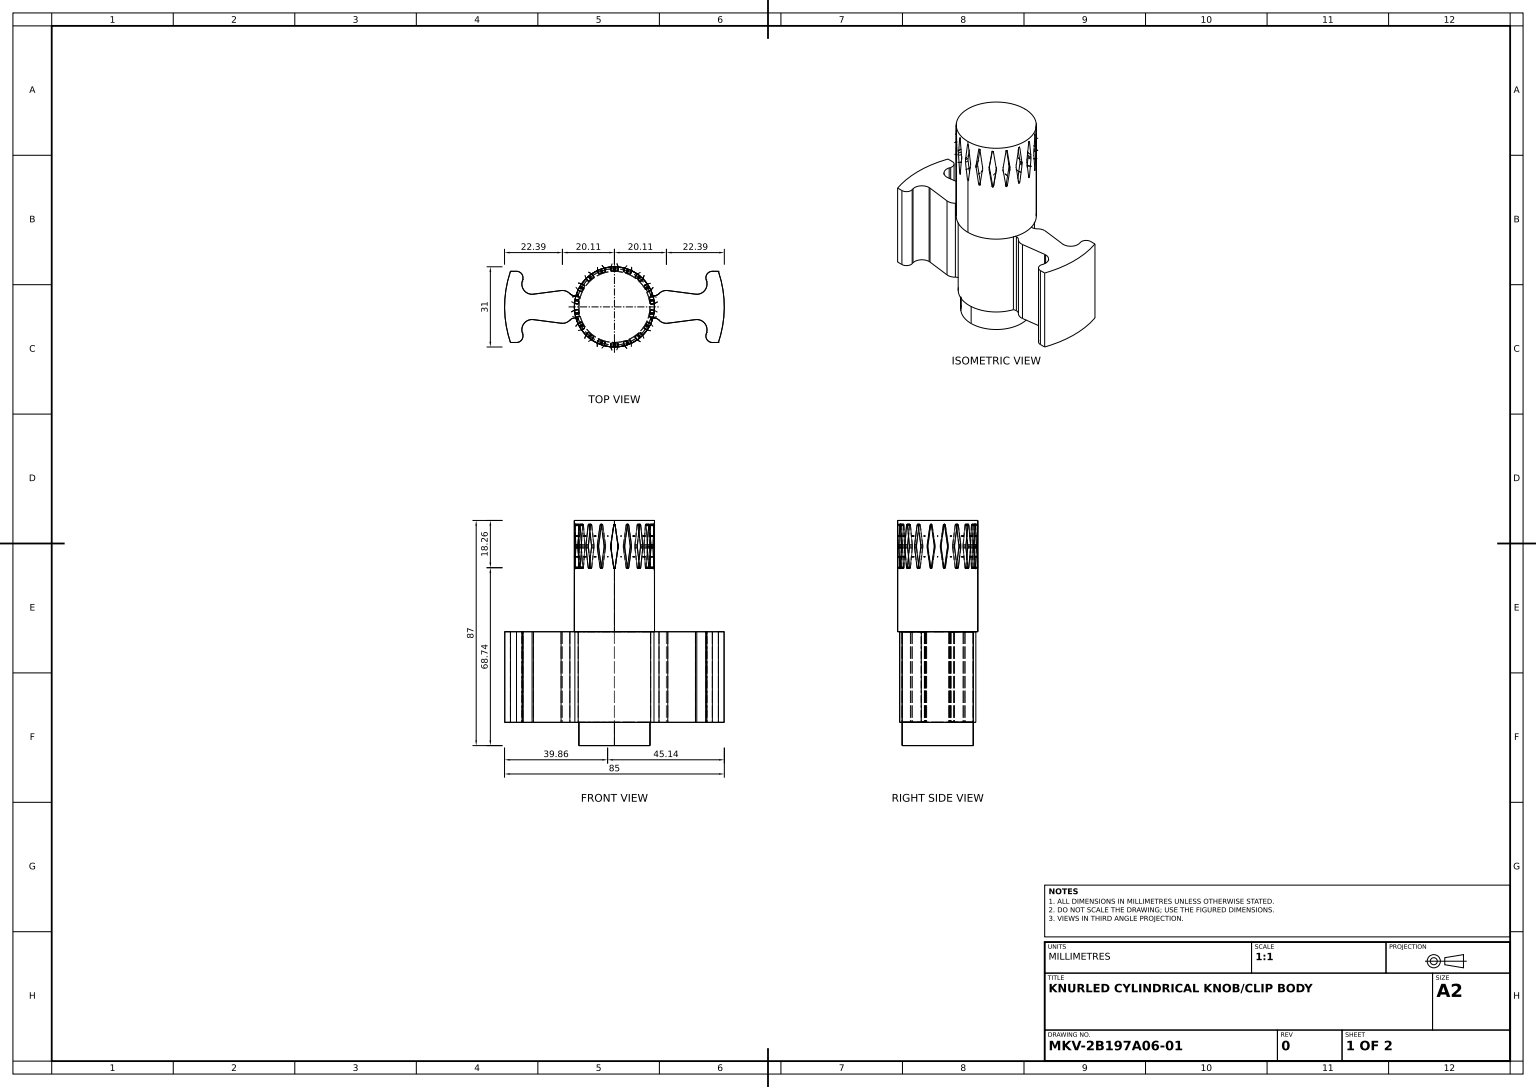
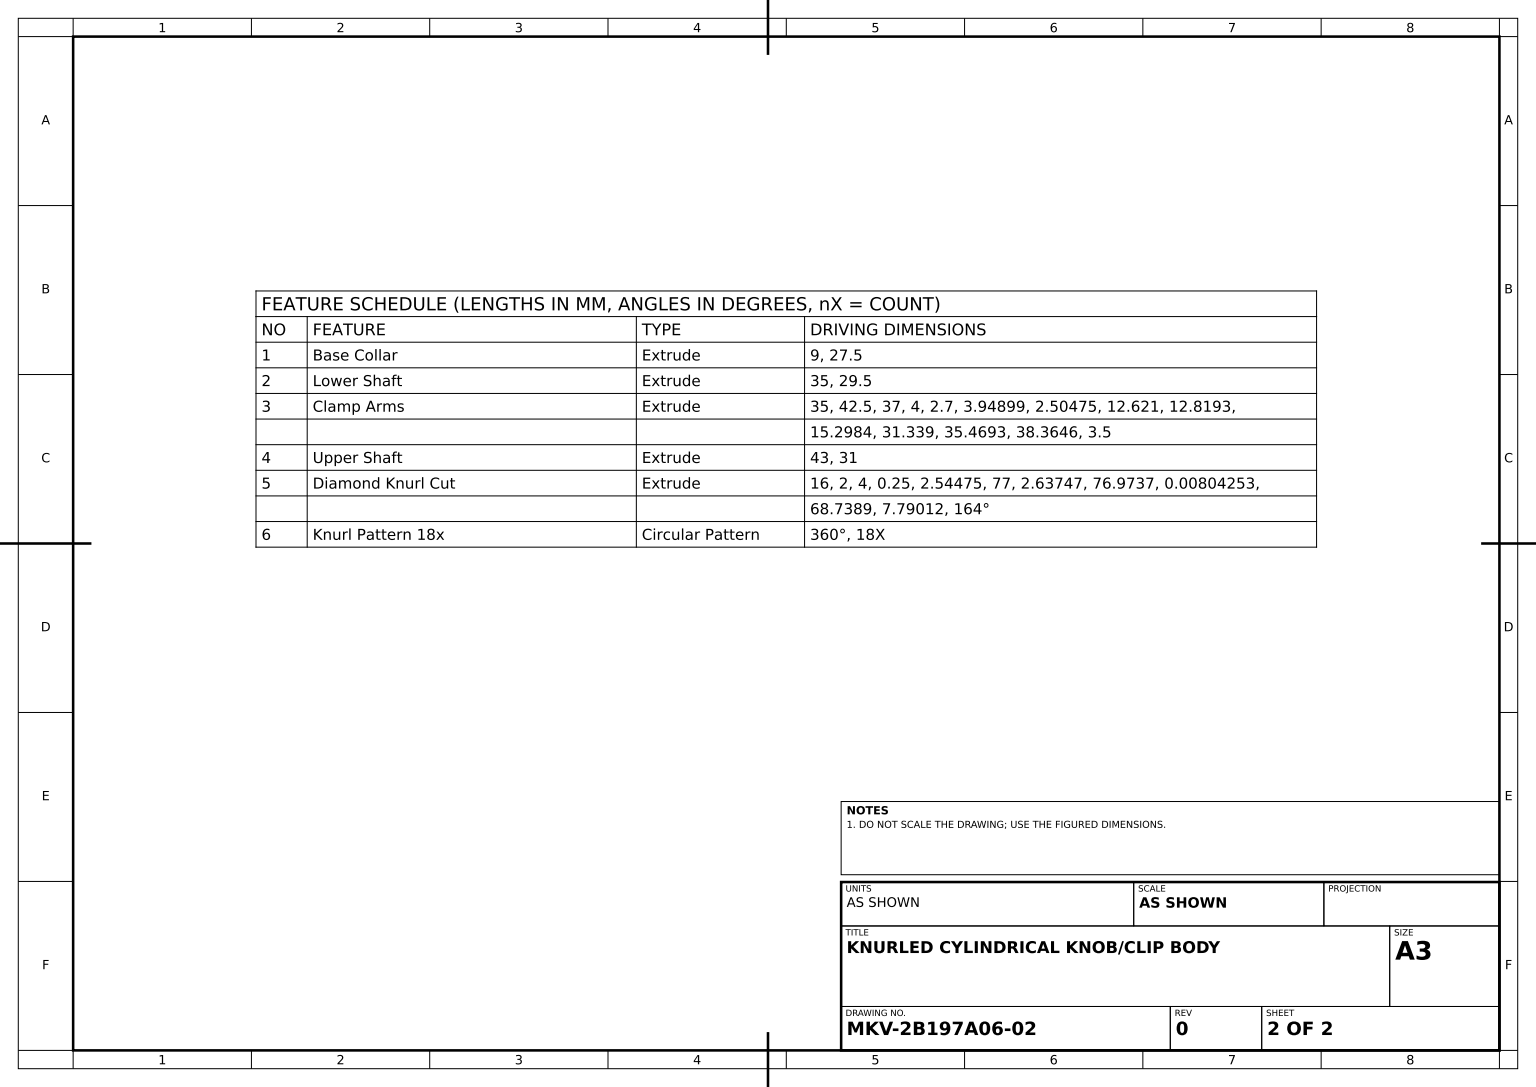
from build123d import *

# Parameters (mm, degrees)
BASE_COLLAR_SKETCH_R    = 13.75
BASE_COLLAR_DEPTH       = 9
LOWER_SHAFT_SKETCH_R    = 14.75
LOWER_SHAFT_DEPTH       = 35
CLAMP_ARMS_DEPTH        = 35
UPPER_SHAFT_SKETCH_R    = 15.5
UPPER_SHAFT_DEPTH       = 43
DIAMOND_KNURL_CUT_DEPTH = 2
KNURL_PATTERN_18X_COUNT = 18


with BuildPart() as part:
    # Base Collar Sketch → Base Collar (new body)
    with BuildSketch(Plane(origin=(0, 0, 0), x_dir=(1, 0, 0), z_dir=(0, 1, 0))):
        with Locations(Location((0, 0, 0), (0, 0, 270))):
            Circle(BASE_COLLAR_SKETCH_R)
    extrude(amount=BASE_COLLAR_DEPTH)

    # Lower Shaft Sketch → Lower Shaft (add)
    with BuildSketch(Plane(origin=(0, 9, 0), x_dir=(1, 0, 0), z_dir=(0, 1, 0))):
        with Locations(Location((0, 0, 0), (0, 0, 270))):
            Circle(LOWER_SHAFT_SKETCH_R)
    extrude(amount=LOWER_SHAFT_DEPTH)

    # Clamp Arms Sketch → Clamp Arms (add)
    with BuildSketch(Plane.XZ.offset(-9)):
        with BuildLine():
            Line((37.870431389, -13.75), (40.214269855, -13.75))
            ThreePointArc((40.214269855, -13.75), (42.5, 0), (40.214269855, 13.75))
            Line((40.214269855, 13.75), (37.870431389, 13.75))
            ThreePointArc((37.870431389, 13.75), (35.862990958, 12.743233464), (35.469303802, 10.532259389))
            ThreePointArc((35.469303802, 10.532259389), (35.563515946, 10.209619659), (35.654793325, 9.886137414))
            ThreePointArc((35.654793325, 9.886137414), (34.831320299, 6.242068845), (31.338961442, 4.915127559))
            Line((31.338961442, 4.915127559), (20.628220903, 6.311217501))
            ThreePointArc((20.628220903, 6.311217501), (18.792751829, 6.121230791), (17.237871609, 5.127556211))
            ThreePointArc((17.237871609, 5.127556211), (15.702646269, 4.336375699), (14.001999226, 4.637512015))
            ThreePointArc((14.001999226, 4.637512015), (14.75, 0), (14.001999226, -4.637512015))
            ThreePointArc((14.001999226, -4.637512015), (15.702646269, -4.336375699), (17.237871609, -5.127556211))
            ThreePointArc((17.237871609, -5.127556211), (18.792751829, -6.121230791), (20.628220903, -6.311217501))
            Line((20.628220903, -6.311217501), (31.338961442, -4.915127559))
            ThreePointArc((31.338961442, -4.915127559), (34.831320299, -6.242068845), (35.654793325, -9.886137414))
            ThreePointArc((35.654793325, -9.886137414), (35.563515946, -10.209619659), (35.469303802, -10.532259389))
            ThreePointArc((35.469303802, -10.532259389), (35.862990958, -12.743233464), (37.870431389, -13.75))
        make_face()
        with BuildLine():
            ThreePointArc((-17.237871609, -5.127556211), (-15.702646269, -4.336375699), (-14.001999226, -4.637512015))
            ThreePointArc((-14.001999226, -4.637512015), (-14.75, 0), (-14.001999226, 4.637512015))
            ThreePointArc((-14.001999226, 4.637512015), (-15.702646269, 4.336375699), (-17.237871609, 5.127556211))
            ThreePointArc((-17.237871609, 5.127556211), (-18.792751829, 6.121230791), (-20.628220903, 6.311217501))
            Line((-20.628220903, 6.311217501), (-31.338961442, 4.915127559))
            ThreePointArc((-31.338961442, 4.915127559), (-34.831320299, 6.242068845), (-35.654793325, 9.886137414))
            ThreePointArc((-35.654793325, 9.886137414), (-35.563515946, 10.209619659), (-35.469303802, 10.532259389))
            ThreePointArc((-35.469303802, 10.532259389), (-35.862990958, 12.743233464), (-37.870431389, 13.75))
            Line((-37.870431389, 13.75), (-40.214269855, 13.75))
            ThreePointArc((-40.214269855, 13.75), (-42.5, 0), (-40.214269855, -13.75))
            Line((-40.214269855, -13.75), (-37.870431389, -13.75))
            ThreePointArc((-37.870431389, -13.75), (-35.862990958, -12.743233464), (-35.469303802, -10.532259389))
            ThreePointArc((-35.469303802, -10.532259389), (-35.563515946, -10.209619659), (-35.654793325, -9.886137414))
            ThreePointArc((-35.654793325, -9.886137414), (-34.831320299, -6.242068845), (-31.338961442, -4.915127559))
            Line((-31.338961442, -4.915127559), (-20.628220903, -6.311217501))
            ThreePointArc((-20.628220903, -6.311217501), (-18.792751829, -6.121230791), (-17.237871609, -5.127556211))
        make_face()
    extrude(amount=-CLAMP_ARMS_DEPTH)

    # Upper Shaft Sketch → Upper Shaft (add)
    with BuildSketch(Plane(origin=(0, 44, 0), x_dir=(1, 0, 0), z_dir=(0, 1, 0))):
        with Locations(Location((0, 0, 0), (0, 0, 163.745659811))):
            Circle(UPPER_SHAFT_SKETCH_R)
    extrude(amount=UPPER_SHAFT_DEPTH)

    # Diamond Knurl Sketch → Diamond Knurl Cut (cut)
    with BuildSketch(Plane.XY.offset(16)):
        with BuildLine():
            Line((1.323598875, 76.416959946), (0.239524007, 68.704132593))
            ThreePointArc((0.239524007, 68.704132593), (-0.006886298, 68.488931932), (-0.255276622, 68.701844145))
            Line((-0.255276622, 68.701844145), (-1.410995728, 76.406638188))
            ThreePointArc((-1.410995728, 76.406638188), (-1.455250317, 77), (-1.410995728, 77.593361812))
            Line((-1.410995728, 77.593361812), (-0.255405251, 85.297298324))
            ThreePointArc((-0.255405251, 85.297298324), (-0.007462736, 85.509744404), (0.238339671, 85.294825804))
            Line((0.238339671, 85.294825804), (1.324023835, 77.527421342))
            ThreePointArc((1.324023835, 77.527421342), (1.362533929, 76.972175825), (1.323598875, 76.416959946))
        make_face()
    diamond_knurl_cut = extrude(amount=-DIAMOND_KNURL_CUT_DEPTH, mode=Mode.SUBTRACT)

    # Knurl Pattern 18x: Diamond Knurl Cut ×18 about axis
    knurl_pattern_18x_axis = Axis((0, 0, 0), (0, 1, 0))
    for i in range(1, KNURL_PATTERN_18X_COUNT):
        add(diamond_knurl_cut.rotate(knurl_pattern_18x_axis, i * 360 / KNURL_PATTERN_18X_COUNT), mode=Mode.SUBTRACT)


solid = part.part
